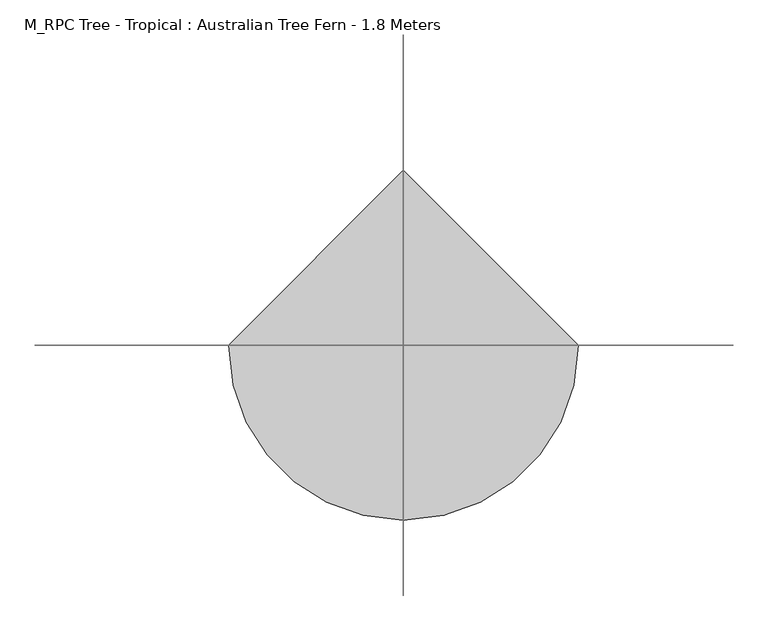
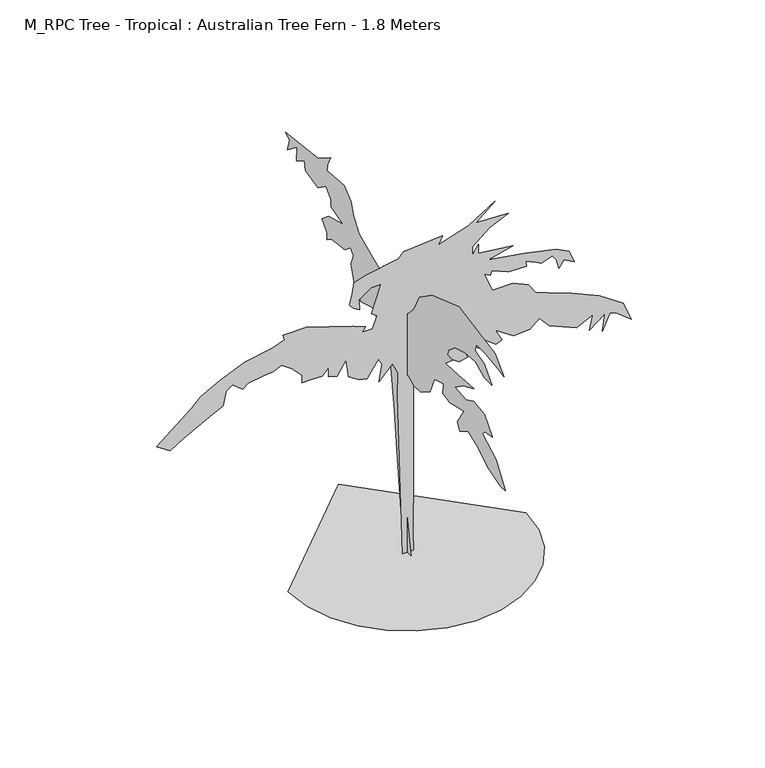
"""IFC4 building model written with IfcOpenShell, lengths in millimetres: geographic element geometry, M_RPC Tree - Tropical : Australian Tree Fern - 1.8 Meters."""

from ifc_helpers import new_model, si_unit, origin, place, context, project, spatial, triangles, source, transform, mapped, element, save


def m_rpc_tree_tropical_australian_tree_fern_1_8_meters_0203a3dd(model_context):
    return source(origin(), model_context, "Body", "Tessellation", [
        triangles([(-628.7763731, 0.0, 0.0007046), (-612.1463562, -144.1188648, 0.0007046), (-564.7912525, -276.4677177, 0.0007046), (-490.4986942, -393.2578274, 0.0007046), (-393.0611461, -490.6953755, 0.0007046), (-276.2710546, -564.9879338, 0.0007046), (-143.9221926, -612.3430012, 0.0007046), (0.1966986, -628.9730181, 0.0007046), (144.3155371, -612.345472, 0.0007046), (276.6643809, -564.9879338, 0.0007046), (393.4545087, -490.6953755, 0.0007046), (490.8920568, -393.2578274, 0.0007046), (565.1846151, -276.4677177, 0.0007046), (612.5396461, -144.1188648, 0.0007046), (629.169663, 5.5e-05, 0.0007046), (0.1965886, 628.9730181, 0.0007046), (463.0895388, -3.44e-05, 1800.0014671), (362.9519737, -2.93e-05, 1714.1689156), (534.6171132, -2.89e-05, 1707.0162998), (434.4795118, -2.61e-05, 1660.5237888), (345.0694533, -2.17e-05, 1585.4212509), (345.0694533, -1.89e-05, 1538.9287399), (377.2569872, -2.19e-05, 1588.9963234), (377.2569872, -1.89e-05, 1538.9287399), (559.6521403, -1.76e-05, 1517.4711834), (430.9020412, -1.57e-05, 1485.2837585), (624.0246283, -1.38e-05, 1453.0961884), (788.537261, -1.16e-05, 1417.333691), (856.4873285, -9.5e-06, 1381.5685776), (885.0973555, -5.5e-06, 1313.6185101), (827.8773016, -7.4e-06, 1345.8060802), (802.8422745, -5e-06, 1306.4660397), (788.537261, -8.2e-06, 1360.111021), (767.0797771, -9.9e-06, 1388.721048), (709.8571798, -8.7e-06, 1367.2636368), (681.2472256, -9.5e-06, 1381.5685776), (627.6021715, -1.1e-05, 1406.6036774), (631.1771713, -9.3e-06, 1377.9936504), (588.2621673, -9.3e-06, 1377.9936504), (534.6171132, -9.5e-06, 1381.5685776), (445.2095255, -1.16e-05, 1417.333691), (441.6320186, -1.01e-05, 1392.2985912), (409.444521, -1.12e-05, 1410.1810753), (452.3620322, -5e-06, 1306.4660397), (559.6521403, -5e-06, 1306.4660397), (641.907185, -2.9e-06, 1270.7035423), (677.6696823, 3e-07, 1217.0584883), (742.04475, 1.8e-06, 1192.0234612), (870.792342, 4.8e-06, 1141.9534069), (1017.4224907, 8.6e-06, 1077.5808826), (1142.5950829, 1.37e-05, 991.7482584), (1185.5101233, 1.99e-05, 888.0332228), (1103.2550423, 1.61e-05, 952.4082905), (1071.0674721, 1.56e-05, 959.5607609), (1031.7275042, 2.08e-05, 873.7282093), (1046.0325176, 1.52e-05, 966.7133039), (963.7774366, 1.91e-05, 902.340707), (981.6599207, 1.42e-05, 984.595788), (895.8273691, 1.67e-05, 941.6782768), (752.7747637, 1.31e-05, 1002.4782721), (699.1297096, 9.5e-06, 1063.2758692), (649.0596554, 1.2e-05, 1020.3582853), (563.2271401, 1.24e-05, 1013.2058149), (466.6670457, 8.6e-06, 1077.5808826), (502.4295794, 1.24e-05, 1013.2058149), (470.2420455, 1.33e-05, 998.9008015), (320.0369333, 6.5e-06, 1113.34338), (413.022028, 1.42e-05, 984.595788), (280.6968927, 8.6e-06, 1077.5808826), (320.0369333, 1.46e-05, 977.4433176), (273.544386, 1.5e-05, 970.2907745), (187.7115619, 1.14e-05, 1031.088299), (87.5742421, 9.5e-06, 1063.2758692), (191.2880696, 1.5e-05, 970.2907745), (30.352694, 1.1e-05, 1038.2408421), (33.9289474, 1.54e-05, 963.1383041), (33.9289474, 3.27e-05, 673.4530066), (33.9289474, 4.76e-05, 423.1103293), (30.352694, 6.66e-05, 104.8153318), (33.9289474, 7.24e-05, 0.0013067), (-23.2925485, 7.27e-05, 0.0006893), (-51.903368, 1.95e-05, 895.1882366), (-48.3268649, 1.2e-05, 1020.3582853), (-76.9376367, 8.4e-06, 1081.1558825), (-148.4644481, 1.29e-05, 1006.0532719), (-134.1591893, 7.3e-06, 1099.0383665), (-152.0409467, 5.4e-06, 1131.2259367), (-180.6514732, 7.8e-06, 1091.8858961), (-212.8384984, 1.05e-05, 1045.3933125), (-252.178539, 1.01e-05, 1052.5458555), (-309.4010636, 8e-06, 1088.3083529), (-323.7060771, 2e-06, 1188.4459179), (-370.1986244, 6.5e-06, 1113.34338), (-416.6911354, 5.6e-06, 1127.6483934), (-416.6911354, 2.6e-06, 1177.7184477), (-448.8761621, 4.8e-06, 1141.9534069), (-509.6737229, 4.8e-06, 1141.9534069), (-556.1662703, 4.8e-06, 1141.9534069), (-556.1662703, 2.2e-06, 1184.8709181), (-609.8138678, -1e-06, 1238.5159721), (-663.4563784, -3.3e-06, 1277.8560127), (-709.9488894, -2e-06, 1256.3984562), (-760.0189436, -1.8e-06, 1252.8210583), (-842.2740246, -1e-06, 1238.5159721), (-870.8865223, 3e-07, 1217.0584883), (-924.5315763, -2.3e-06, 1259.9735287), (-956.7166031, -8e-07, 1234.9384289), (-974.5991598, 3.7e-06, 1159.8359636), (-1074.7367249, 6.7e-06, 1109.7683802), (-1185.6043036, 1.03e-05, 1048.9708557), (-1253.5542984, 1.29e-05, 1006.0532719), (-1325.0819092, 1.01e-05, 1052.5458555), (-1139.1117926, 1.2e-06, 1202.7534748), (-1092.6192089, -1.8e-06, 1252.8210583), (-992.4816439, -5e-06, 1306.4660397), (-860.1565086, -8.4e-06, 1363.6885643), (-709.9488894, -1.01e-05, 1392.2985912), (-649.1513649, -1.14e-05, 1413.7561478), (-656.303908, -1.31e-05, 1442.3661747), (-531.1337502, -1.31e-05, 1442.3661747), (-409.5361579, -1.08e-05, 1403.0286049), (-287.9410727, -8.4e-06, 1363.6885643), (-219.9912595, -6.9e-06, 1338.6536098), (-237.873035, -5.5e-06, 1313.6185101), (-184.2277266, -5.5e-06, 1313.6185101), (-159.1934625, -9.3e-06, 1377.9936504), (-187.8042343, -1.06e-05, 1399.4510616), (-137.7354336, -1.93e-05, 1546.0812103), (-191.3804877, -1.93e-05, 1546.0812103), (-255.7535388, -1.65e-05, 1499.5886993), (-252.178539, -1.31e-05, 1442.3661747), (-284.3660728, -1.44e-05, 1463.826202), (-305.8235567, -1.59e-05, 1488.8586857), (-291.5185614, -1.91e-05, 1542.5036671), (-280.7885659, -2.27e-05, 1603.303735), (-216.4150061, -2.4e-05, 1624.7612915), (-44.7506115, -2.59e-05, 1656.9488617), (-19.7161203, -2.76e-05, 1685.5588886), (187.7115619, -2.87e-05, 1703.4413727), (166.2535512, -2.61e-05, 1660.5237888), (323.6119331, -2.91e-05, 1710.5938431), (0.1967009, -848.2856489, 1525.4262211), (0.1966947, -721.9905962, 1545.7961987), (0.1966909, -636.4380421, 1545.7961987), (0.1966914, -620.1404903, 1505.0562435), (0.1966961, -709.7680864, 1480.611224), (0.1967013, -774.9531338, 1403.206065), (0.1966982, -705.6955879, 1403.206065), (0.1966934, -624.2155323, 1443.9461655), (0.1966894, -530.5129306, 1435.7960815), (0.1966861, -436.812836, 1407.2786362), (0.196685, -379.7777999, 1358.3910679), (0.1966854, -367.5552901, 1325.7985806), (0.1966876, -416.4428221, 1325.7985806), (0.1966864, -351.2577747, 1268.7635445), (0.1966897, -428.6653318, 1272.8385864), (0.1966975, -611.9930225, 1285.0610962), (0.1966943, -510.1429167, 1240.2459538), (0.1966926, -436.812836, 1187.2834162), (0.1966974, -538.6629418, 1179.1359484), (0.1966995, -607.9204877, 1211.7284357), (0.1967043, -705.6955879, 1199.5059259), (0.1967102, -783.1006016, 1118.0258703), (0.1967074, -713.8430557, 1105.805904), (0.1967071, -689.4005796, 1081.3608845), (0.1967146, -811.6181196, 1012.1033386), (0.1967223, -901.2457157, 889.8831825), (0.1967202, -852.3581474, 885.810684), (0.1967138, -734.213106, 922.4757425), (0.1967074, -632.3630001, 983.5858206), (0.1967032, -559.0329557, 1016.1783079), (0.1967012, -481.6253986, 967.2882689), (0.1966991, -461.2553847, 1008.0282967), (0.1966989, -522.3654264, 1105.805904), (0.196694, -391.9978025, 1073.213344), (0.1966907, -326.8152623, 1085.4358538), (0.1966892, -330.8877608, 1142.4708899), (0.1966863, -249.4091949, 1118.0258703), (0.1966873, -208.6694215, 1024.3258484), (0.1966852, -127.189602, 971.3633108), (0.1966824, -62.006049, 967.2882689), (0.1966794, -13.1181855, 995.8083303), (0.1966778, 31.6955263, 983.5858206), (0.1966755, 52.0655402, 1028.3983469), (0.1966759, 80.5833171, 971.3633108), (0.1966779, 84.6573144, 898.030723), (0.1966865, 56.1395466, 653.5930269), (0.1966983, 19.473666, 311.3777598), (0.1967098, -33.4880268, 0.0007036), (0.1967069, 35.7695282, 0.0), (0.1967013, 52.0655402, 164.7148733), (0.1966905, 88.7315752, 470.2628654), (0.1966817, 117.2490932, 722.8505728), (0.1966725, 153.9151146, 975.4382801), (0.1966664, 206.8769073, 1101.730862), (0.1966639, 263.9127065, 1101.730862), (0.1966599, 300.5777468, 1179.1359484), (0.1966575, 365.762776, 1162.8409401), (0.1966555, 422.7978484, 1142.4708899), (0.196651, 483.9078901, 1203.5809679), (0.1966468, 512.4254082, 1301.3560318), (0.196646, 492.0553943, 1358.3910679), (0.1966439, 520.5729123, 1386.9086586), (0.1966429, 569.4604443, 1346.1685581), (0.1966379, 691.6805277, 1329.8736225), (0.196637, 732.4205555, 1301.3560318), (0.1966357, 732.4205555, 1342.0961323), (0.1966321, 781.3081238, 1390.9835552), (0.1966334, 720.1980457, 1439.8711235), (0.1966381, 589.8304582, 1476.536182), (0.1966324, 695.7555696, 1509.1286694), (0.1966311, 699.8280682, 1545.7961987), (0.1966277, 744.6430653, 1594.6837669), (0.196626, 817.9731823, 1541.721302), (0.1966201, 932.0457253, 1566.1637054), (0.1966183, 940.1932657, 1615.0537445), (0.1966162, 1013.5257809, 1574.3137894), (0.1966141, 1009.4508116, 1651.718803), (0.1966123, 1095.0059092, 1586.5338284), (0.1966112, 1078.7083574, 1647.6437611), (0.1966088, 1115.3758867, 1672.0887806), (0.1966211, 817.9731823, 1704.6814133), (0.196624, 703.9030375, 1778.011385), (0.1966245, 728.3455862, 1725.0513908), (0.1966254, 736.4955975, 1684.3112904), (0.196632, 577.6079484, 1700.6063713), (0.1966365, 512.4254082, 1647.6437611), (0.1966393, 492.0553943, 1582.4612572), (0.1966437, 439.0928567, 1513.2037113), (0.1966509, 316.875244, 1456.1662045), (0.1966608, 141.6931136, 1386.9086586), (0.1966549, 223.1726787, 1464.316143), (0.1966615, 113.1750868, 1407.2786362), (0.1966689, -0.8962257, 1329.8736225), (0.1966697, -62.006049, 1395.0585972), (0.1966689, -110.8938398, 1492.8337337), (0.1966718, -229.039181, 1574.3137894), (0.1966802, -473.4778945, 1659.8662708), (0.196691, -689.4005796, 1619.1263157), (0.1966968, -803.4706518, 1598.7563381), (0.1967028, -884.9507074, 1517.2762825)], [[15, 16, 1], [14, 15, 1], [14, 1, 2], [13, 14, 2], [13, 2, 3], [13, 3, 4], [12, 13, 4], [11, 12, 4], [11, 4, 5], [11, 5, 6], [11, 6, 7], [11, 7, 8], [11, 8, 9], [11, 9, 10], [141, 17, 18], [54, 55, 56], [73, 74, 75], [67, 68, 69], [24, 25, 26], [18, 19, 20], [51, 52, 53], [22, 23, 24], [84, 85, 86], [29, 30, 31], [56, 57, 58], [31, 32, 33], [130, 131, 132], [138, 139, 140], [41, 42, 43], [111, 112, 113], [110, 111, 113], [109, 110, 113], [122, 123, 124], [118, 119, 120], [18, 20, 21], [141, 18, 21], [69, 70, 71], [69, 71, 72], [28, 29, 31], [28, 31, 33], [28, 33, 34], [27, 28, 34], [27, 34, 35], [27, 35, 36], [27, 36, 37], [130, 132, 133], [130, 133, 134], [50, 51, 53], [50, 53, 54], [50, 54, 56], [50, 56, 58], [140, 141, 21], [37, 38, 39], [64, 65, 66], [64, 66, 67], [80, 81, 82], [79, 80, 82], [78, 79, 82], [77, 78, 82], [76, 77, 82], [76, 82, 83], [75, 76, 83], [97, 98, 99], [49, 50, 58], [49, 58, 59], [49, 59, 60], [48, 49, 60], [48, 60, 61], [47, 48, 61], [129, 130, 134], [129, 134, 135], [129, 135, 136], [129, 136, 137], [128, 129, 137], [108, 109, 113], [108, 113, 114], [107, 108, 114], [107, 114, 115], [106, 107, 115], [106, 115, 116], [105, 106, 116], [104, 105, 116], [103, 104, 116], [103, 116, 117], [102, 103, 117], [101, 102, 117], [101, 117, 118], [75, 83, 84], [26, 27, 37], [26, 37, 39], [26, 39, 40], [26, 40, 41], [26, 41, 43], [92, 93, 94], [92, 94, 95], [126, 127, 128], [101, 118, 120], [100, 101, 120], [100, 120, 121], [99, 100, 121], [97, 99, 121], [96, 97, 121], [95, 96, 121], [95, 121, 122], [92, 95, 122], [92, 122, 124], [140, 21, 22], [88, 89, 90], [24, 26, 43], [22, 24, 43], [88, 90, 91], [88, 91, 92], [88, 92, 124], [87, 88, 124], [87, 124, 125], [47, 61, 62], [47, 62, 63], [47, 63, 64], [46, 47, 64], [45, 46, 64], [44, 45, 64], [44, 64, 67], [43, 44, 67], [137, 138, 140], [128, 137, 140], [126, 128, 140], [126, 140, 22], [126, 22, 43], [126, 43, 67], [126, 67, 69], [126, 69, 72], [126, 72, 73], [125, 126, 73], [87, 125, 73], [87, 73, 75], [87, 75, 84], [87, 84, 86], [231, 232, 233], [156, 157, 158], [240, 241, 142], [222, 223, 224], [218, 219, 220], [220, 221, 222], [218, 220, 222], [153, 154, 155], [240, 142, 143], [239, 240, 143], [146, 147, 148], [205, 206, 207], [162, 163, 164], [156, 158, 159], [216, 217, 218], [216, 218, 222], [166, 167, 168], [166, 168, 169], [222, 224, 225], [239, 143, 144], [238, 239, 144], [146, 148, 149], [145, 146, 149], [165, 166, 169], [165, 169, 170], [207, 208, 209], [188, 189, 190], [188, 190, 191], [188, 191, 192], [187, 188, 192], [187, 192, 193], [186, 187, 193], [186, 193, 194], [185, 186, 194], [171, 172, 173], [171, 173, 174], [145, 149, 150], [155, 156, 159], [165, 170, 171], [165, 171, 174], [175, 176, 177], [182, 183, 184], [205, 207, 209], [205, 209, 210], [204, 205, 210], [203, 204, 210], [161, 162, 164], [161, 164, 165], [161, 165, 174], [160, 161, 174], [159, 160, 174], [159, 174, 175], [159, 175, 177], [155, 159, 177], [238, 144, 145], [238, 145, 150], [237, 238, 150], [237, 150, 151], [237, 151, 152], [236, 237, 152], [235, 236, 152], [235, 152, 153], [235, 153, 155], [235, 155, 177], [235, 177, 178], [234, 235, 178], [234, 178, 179], [234, 179, 180], [234, 180, 181], [234, 181, 182], [234, 182, 184], [231, 233, 234], [231, 234, 184], [214, 215, 216], [214, 216, 222], [213, 214, 222], [213, 222, 225], [213, 225, 226], [212, 213, 226], [212, 226, 227], [212, 227, 228], [211, 212, 228], [210, 211, 228], [210, 228, 229], [203, 210, 229], [203, 229, 230], [202, 203, 230], [184, 185, 194], [184, 194, 195], [231, 184, 195], [230, 231, 195], [230, 195, 196], [230, 196, 197], [202, 230, 197], [202, 197, 198], [201, 202, 198], [200, 201, 198], [199, 200, 198]], closed=False),
    ])


if __name__ == "__main__":
    model = new_model("IFC4")
    model_context = context("Model", 3, world=origin())
    ifc_project = project(units=[si_unit("LENGTHUNIT", "METRE", prefix="MILLI")], contexts=[model_context])
    site = spatial("IfcSite", under=ifc_project)
    building = spatial("IfcBuilding", under=site)
    placement = place(None, origin())
    m_rpc_tree_tropical_australian_tree_fern_1_8_meters_shape = m_rpc_tree_tropical_australian_tree_fern_1_8_meters_0203a3dd(model_context)
    element("IfcGeographicElement", 1, ObjectType="M_RPC Tree - Tropical : Australian Tree Fern - 1.8 Meters", at=placement, inside=building, context=model_context, shape_type="MappedRepresentation", body=[
        mapped(m_rpc_tree_tropical_australian_tree_fern_1_8_meters_shape, transform((0.0, 0.0, 0.0), x_axis=(1.0, 0.0, 0.0), y_axis=(0.0, 1.0, 0.0), z_axis=(0.0, 0.0, 1.0))),
    ])
    save(model, "model.ifc")

# Revit data of these elements
# Type "M_RPC Tree - Tropical : Australian Tree Fern - 1.8 Meters"
#   built-in parameter 1005198 = "{2, 15},{39, RPC-16-FVCN-UWG0-AP53-A000-ST1L-LVER-AU},{1, 0},{1, 0},{2, 35},{1, 8},{5, Color},{1, 0},{1, 0},{3, 0.8},{3, 0.8},{3, 0.8},{1, 8},{7, BBoxMin},{1, 0},{1, 0},{1, 0},{1, 0},{1, 0},{1, 8},{7, BBoxMax},{1, 0},{1, 0},{1, 0},{1, 0},{1, 0},{2, 11},{9, RPCTypeId},{1, 0},{1, 0},{39, RPC-16-FVCN-UWG0-AP53-A000-ST1L-LVER-AU},{1, 6},{14, RPCPlantHeight},{1, 0},{1, 0},{7, 5.90551},{2, 11},{7, keyword},{1, 0},{1, 0},{99, :Geometry:RPC:Australian Tree Fern:Alsophila cooperi (Cyathea australis):Sydney:Tree fern:Tropical.},{2, 11},{8, category},{1, 0},{1, 0},{17, :Trees [Tropical]},{2, 11},{12, LocalizedUID},{1, 0},{1, 0},{20, Australian Tree Fern},{2, 14},{6, Height},{1, 0},{1, 0},{7, 5.90551},{1, 2},{16, Cast Reflections},{1, 0},{1, 0},{1, 0},{1, 2},{12, Cast Shadows},{1, 0},{1, 0},{1, 1},{1, 2},{9, Lock View},{1, 0},{1, 0},{1, 0},{1, 4},{5, ViewC},{1, 0},{1, 0},{1, 0},{2, 11},{20, AdvancedUIDefinition},{1, 0},{1, 0},{0, },{2, 11},{10, AssetLibID},{1, 0},{1, 0},{36, 4D3F6E72-3F99-4203-98E9-AF80B3C7A7A4},{2, 11},{10, BaseSchema},{1, 0},{1, 0},{9, RPCSchema},{2, 11},{12, ExchangeGUID},{1, 0},{1, 0},{0, },{1, 2},{6, Hidden},{1, 0},{1, 0},{1, 0},{1, 4},{11, RPCCategory},{1, 0},{1, 0},{1, 0},{2, 11},{8, RPCImage},{1, 0},{1, 0},{0, },{1, 4},{13, SchemaVersion},{1, 0},{1, 0},{1, 4},{2, 11},{12, UIDefinition},{1, 0},{1, 0},{0, },{2, 11},{6, UIName},{1, 0},{1, 0},{39, RPC-16-FVCN-UWG0-AP53-A000-ST1L-LVER-AU},{2, 11},{11, VersionGUID},{1, 0},{1, 0},{9, RPCSchema},{2, 11},{9, assettype},{1, 0},{1, 0},{11, RPCGeometry},{2, 11},{11, description},{1, 0},{1, 0},{0, },{2, 11},{9, localname},{1, 0},{1, 0},{3, RPC},{2, 11},{9, localtype},{1, 0},{1, 0},{3, RPC},{1, 4},{8, revision},{1, 0},{1, 0},{1, 1},{2, 11},{9, thumbnail},{1, 0},{1, 0},{0, },{1, 4},{7, version},{1, 0},{1, 0},{1, 1},{1, 2},{20, RPC_Cast Reflections},{1, 0},{1, 0},{1, 1},{1, 2},{16, RPC_Cast Shadows},{1, 0},{1, 0},{1, 1},{1, 2},{13, RPC_Lock View},{1, 0},{1, 0},{1, 0},{1, 4},{9, RPC_ViewC},{1, 0},{1, 0},{1, 0},{21, assetlibrary_base.fbx},{1, 5},"
#   built-in parameter 1005195 = "RPC-16-FVCN-UWG0-AP53-A000-ST1L-LVER-AU"
#   Type Comments = "Australian Tree Fern"
#   Height = 5' - 10.86614"
#   Plan Symbol = element 432532
#   Description = (empty or 0)
#   Default Elevation = 0
